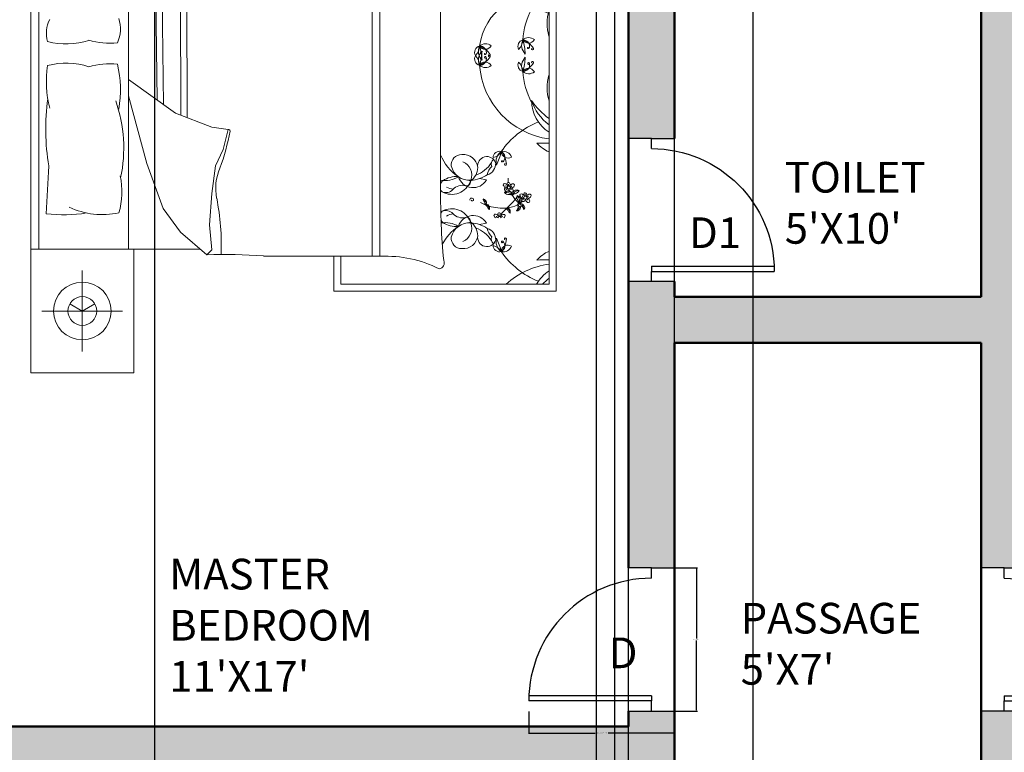
# Model space of a CAD drawing. Units: inches. Extents: x -55 to 413, y -498 to 86.
# Tile 4 of 6: x 45 to 238, y -201 to -57. Entities that reach past the tile are written whole.
import ezdxf

# ---------------------------------------------------------------- set-up
doc = ezdxf.new("R2010")
doc.units = ezdxf.units.IN
doc.header["$MEASUREMENT"] = 0
for name, color, linetype, lineweight in [('A-ANNO-DIMS', 2, 'Continuous', 18), ('A-ANNO-TEXT', 7, 'Continuous', 25), ('A-AREA-IDEN', 7, 'Continuous', 25), ('A-DOOR', 3, 'Continuous', 25), ('A-FURN', 9, 'Continuous', 18), ('A-WALL', 7, 'Continuous', 50), ('A-WALL-PATT', 8, 'Continuous', 13)]:
    doc.layers.add(name, color=color, linetype=linetype, lineweight=lineweight)
doc.styles.get("Standard").update_dxf_attribs({"font": 'arial.ttf'})
doc.dimstyles.get("Standard").update_dxf_attribs({"dimtxt": 0.18, "dimasz": 0.18, "dimexe": 0.18, "dimexo": 0.0625, "dimgap": 0.09, "dimtad": 0, "dimtih": 1, "dimtoh": 1, "dimdec": 0, "dimzin": 0, "dimdsep": 46, "dimlunit": 3, "dimtxsty": 'Standard', "dimcen": 0.09, "dimadec": 0, "dimazin": 0, "dimtfac": 1, "dimtdec": 0, "dimtofl": 0, "dimtmove": 0, "dimatfit": 3, "dimfxl": 1, "dimtolj": 1, "dimtzin": 0, "dimarcsym": 0})

# ---------------------------------------------------------------- blocks, each defined once
blk = doc.blocks.new('BED-DOUBLE-WITH-NIGHTSTANDS')
for p, q in [((0, 0), (0, 120.84)), ((10.07, 100.86), (10.07, 116.65)), ((17.96, 108.75), (2.18, 108.75)), ((59.24, 97.34), (59.24, 104.05)), ((59.24, 104.05), (102.77, 104.05)), ((102.77, 104.05), (102.77, 15.95)), ((60.64, 102.65), (60.64, 97.32)), ((101.37, 102.65), (60.64, 102.65)), ((101.37, 17.35), (101.37, 102.65)), ((1.55, 96.67), (1.55, 24.17)), ((19.1, 24.17), (19.1, 96.67)), ((24.12, 96.35), (24.72, 53.32)), ((25.36, 96.3), (25.98, 52.42)), ((66.77, 97.22), (66.77, 22.78)), ((68.28, 97.33), (68.28, 22.78)), ((29.16, 96.24), (29.34, 50.35)), ((30.4, 96.24), (30.59, 49.88)), ((89.11, 90.74), (87.75, 91)), ((80.15, 84.95), (80.15, 35.89)), ((89.11, 82.29), (87.75, 82.03)), ((19.1, 57.36), (28.31, 50.74)), ((22.69, 40.95), (19.1, 54.13)), ((28.31, 50.74), (35.41, 48.05)), ((35.41, 48.05), (38.59, 47.56)), ((38.59, 47.56), (37.61, 43.64)), ((37.61, 43.64), (36.14, 40.46)), ((25.87, 32.14), (22.69, 40.95)), ((36.14, 40.46), (35.41, 35.08)), ((89.11, 37.7), (87.75, 37.97)), ((35.41, 35.08), (34.92, 28.96)), ((29.29, 27.49), (25.87, 32.14)), ((34.92, 28.96), (35.41, 24.06)), ((89.11, 29.26), (87.75, 28.99)), ((34.43, 23.09), (29.29, 27.49)), ((0, 24.17), (33.17, 24.17)), ((35.41, 24.06), (34.43, 23.09)), ((59.24, 15.95), (59.24, 22.78)), ((60.64, 22.78), (60.64, 17.35)), ((10.07, 19.98), (10.07, 4.19)), ((60.64, 17.35), (101.37, 17.35)), ((102.77, 15.95), (59.24, 15.95)), ((17.96, 12.08), (2.18, 12.08))]:
    blk.add_line(p, q)
for points in [[(0, 96.67), (20.14, 96.67), (20.14, 120.84), (0, 120.84)], [(10.07, 108.75), (7.63, 107.35)], [(10.07, 108.75), (12.51, 107.35)], [(20.14, 24.17), (20.14, 0), (0, 0)], [(10.07, 12.08), (7.63, 13.49)], [(10.07, 12.08), (12.51, 13.49)]]:
    blk.add_lwpolyline(points)
for points in [[(65.82, 97.19, 0.056112), (72.47, 98.06, 0.095341), (78.87, 99.76)], [(3.01, 89.73, -0.074897), (10.9, 89.58, 0.472817)], [(11.35, 65.01, -0.14099), (3.29, 64.77, -0.235245)], [(11.35, 59.85, 0.14099), (3.29, 60.09, 0.235245)], [(3.01, 31.11, 0.074897), (10.9, 31.25, -0.472817)], [(45.49, 22.83, 0.001242), (68.42, 22.78, -0.127202), (79.85, 20.35)]]:
    blk.add_lwpolyline(points, format="xyb")
for centre, radius in [((10.07, 108.75), 5.64), ((10.07, 108.75), 2.82), ((96.74, 85.77), 0.308), ((93.49, 83.76), 0.308), ((93.49, 36.24), 0.308), ((96.74, 34.23), 0.308), ((10.07, 12.08), 5.64), ((10.07, 12.08), 2.82)]:
    blk.add_circle(centre, radius)
for centre, radius, start, end in [((105.05, 87.4), 15.78, 111.4092, 145.6135), ((103.49, 114.39), 15.78, 228.1144, 262.255), ((105.6, 106.48), 7.69, 209.8884, 236.5383), ((107.04, 109.24), 9.58, 223.5186, 233.6964), ((79.49, 98.85), 1.1, 336.5219, 123.8264), ((197.68, 88.65), 117.59, 175.2402, 181.8035), ((33.86, 313.3), 217.13, 266.1, 270.9282), ((41.76, 379.4), 283.23, 269.1145, 274.8735), ((91.72, 95.04), 1.31, 76.272, 177.0484), ((89.73, 97.71), 2.7, 284.7031, 328.6173), ((93.49, 94.28), 2.49, 125.7657, 194.5347), ((81.25, 98.7), 11.04, 332.8176, 347.4827), ((92.4, 94.6), 1.75, 20.9613, 102.2885), ((93.35, 96.35), 1.32, 181.7131, 301.5367), ((89.03, 93.68), 3.99, 2.0648, 41.1598), ((91.43, 95.17), 1.29, 316.2238, 62.3173), ((103.83, 102.17), 6.42, 221.0454, 247.4453), ((100.38, 119.75), 21.83, 266.3481, 272.5919), ((88.66, 99), 9.15, 203.6453, 236.3329), ((84.27, 93.67), 2.04, 88.9462, 185.5144), ((84.56, 92.84), 2.89, 7.1143, 95.0551), ((89.21, 93.5), 1.81, 19.1312, 189.736), ((91.18, 93.88), 1.11, 126.7319, 206.0245), ((92.17, 94.41), 0.103, 20.2667, 316.2271), ((85.78, 94.3), 3.63, 193.079, 274.7067), ((83.46, 91.7), 2.8, 338.5779, 68.4181), ((83.92, 93.34), 3.51, 305.9599, 357.6409), ((85.22, 97.1), 5.7, 288.2955, 328.7386), ((88.67, 93.94), 2.26, 285.6955, 4.031), ((91.68, 91.5), 2.41, 128.4175, 173.8338), ((92.82, 93.82), 0.196, 168.5166, 2.0648), ((92.72, 93.84), 0.0952, 52.0591, 168.5166), ((81.49, 89.45), 1.46, 127.675, 162.5814), ((81.04, 95.65), 5.01, 259.249, 301.1782), ((83.22, 86.74), 4.66, 85.2696, 124.215), ((86.51, 92.24), 3, 196.8663, 330.0915), ((83.22, 86.74), 4.66, 53.6555, 57.2989), ((85.68, 97.15), 6.48, 273.4924, 303.7117), ((-1146.98, 23.12), 1151.92, 2.85022, 3.31479), ((14.07, 74.34), 15.57, 78.2417, 114.8684), ((1.6, 85.42), 16.19, 348.9631, 14.8961), ((81.49, 89.45), 1.46, 196.6343, 225.5483), ((82.34, 91.77), 3.85, 240.8249, 340.7178), ((81.2, 90.06), 1.81, 246.1646, 318.4347), ((83.04, 92.35), 3.47, 240.0851, 262.564), ((84.4, 87.22), 2.48, 74.8529, 138.4347), ((85.25, 90.33), 0.75, 254.8529, 12.6959), ((90.82, 89.21), 0.238, 125.0752, 284.7644), ((91.19, 89.3), 0.513, 127.3642, 168.4363), ((90.79, 89.71), 0.74, 277.4968, 341.2737), ((91.37, 89.36), 0.294, 88.1325, 178.8919), ((91.96, 89.05), 0.636, 136.3462, 189.6513), ((91.6, 88.99), 0.265, 189.6513, 312.3208), ((91.66, 89.72), 0.308, 183.2768, 356.7232), ((92.63, 89.17), 1.01, 164.2829, 186.9148), ((91.44, 89.17), 0.504, 312.3208, 40.2111), ((92.5, 89.73), 0.715, 201.6382, 274.947), ((91.56, 88.75), 0.934, 42.3896, 66.5724), ((100.98, 96.15), 11.47, 217.9541, 226.8459), ((92.23, 89.3), 0.508, 10.9597, 52.2379), ((92.55, 89.26), 0.236, 274.947, 37.5263), ((94.05, 88.22), 0.634, 115.5379, 168.6744), ((91.9, 89.14), 1.91, 329.344, 349.7412), ((90.37, 88.7), 3.41, 352.8698, 1.6736), ((92.47, 77.79), 10.01, 110.1059, 116.9968), ((86.93, 87.31), 1.94, 336.3901, 344.4871), ((89.04, 86.81), 0.246, 83.9457, 185.6216), ((88.06, 87.04), 1.01, 328.836, 0.8141), ((88.58, 86.75), 0.58, 306.5232, 32.4668), ((89.27, 87.2), 0.246, 112.5583, 214.2343), ((89.11, 87.64), 0.58, 265.7131, 351.6568), ((88.6, 87.96), 1.01, 297.3659, 329.344), ((87.84, 88.83), 1.94, 313.6929, 321.7899), ((89.98, 87.5), 0.634, 115.5379, 168.6744), ((87.83, 88.42), 1.91, 329.344, 349.7412), ((92.47, 77.79), 10.01, 86.1723, 106.4158), ((86.31, 87.98), 3.41, 352.8698, 1.6736), ((93.34, 87.92), 0.246, 112.5583, 214.2343), ((93.18, 88.36), 0.58, 265.7131, 351.6568), ((92.67, 88.68), 1.01, 297.3659, 329.344), ((92.72, 82.78), 5.02, 60.7959, 85.244), ((82.04, 75.56), 16.51, 37.8256, 47.7588), ((91.9, 89.55), 1.94, 313.6929, 321.7899), ((99.38, 82.26), 6.02, 130.182, 149.456), ((95.16, 88.01), 0.344, 33.0979, 123.1364), ((87.59, 83.16), 8.99, 31.1156, 34.8118), ((94.67, 87.42), 0.93, 2.3172, 70.5201), ((94.22, 86.41), 1.4, 310.9365, 22.7695), ((95.43, 87.19), 0.268, 135.7354, 318.1297), ((94.99, 87.63), 0.356, 315.7354, 31.1156), ((94.69, 86.87), 0.826, 319.3812, 5.5456), ((95.64, 87.19), 0.268, 68.2452, 250.6395), ((95.02, 87.52), 0.801, 352.6008, 57.1845), ((97.88, 82.14), 5.36, 111.7087, 116.2181), ((92.72, 82.78), 5.02, 47.5083, 55.9967), ((95.78, 87.7), 0.801, 252.8042, 349.6943), ((95.02, 86.27), 0.853, 331.1838, 51.6792), ((95.87, 87.77), 0.356, 248.2452, 323.6254), ((95.55, 87.99), 0.93, 291.7087, 3.0299), ((88.91, 92.89), 8.99, 323.6254, 327.3216), ((96.29, 87.75), 0.344, 325.6077, 55.6462), ((97.67, 85.85), 0.97, 121.9501, 165.2442), ((97.31, 86.42), 0.305, 44.3732, 121.9501), ((82.34, 81.26), 3.85, 19.2822, 119.1751), ((81.2, 82.97), 1.81, 41.5653, 113.8354), ((86.24, 86.19), 0.379, 169.5864, 349.5616), ((86.38, 86.17), 0.233, 349.5616, 167.2949), ((89.11, 86.04), 0.634, 129.5056, 182.6421), ((87.29, 87.51), 1.91, 308.4388, 328.836), ((86.96, 89.06), 3.41, 296.5064, 305.3102), ((93.04, 86.11), 1.4, 253.6301, 325.4631), ((93.43, 84.17), 0.992, 82.0748, 142.6895), ((93.32, 85.53), 1.02, 228.342, 274.9894), ((93.35, 85.36), 0.853, 273.8774, 357.1501), ((93.68, 85.97), 0.826, 262.0748, 308.2393), ((95.01, 85.12), 0.853, 181.4625, 249.4747), ((94.87, 85.79), 0.826, 215.1128, 261.2773), ((95.53, 85.75), 1.4, 197.889, 269.722), ((94.59, 84), 0.992, 20.6625, 81.2773), ((96.07, 85.69), 0.992, 139.3812, 199.9959), ((94.86, 86.33), 1.02, 285.6484, 332.2957), ((95.89, 85.25), 0.238, 125.0752, 284.7644), ((96.26, 85.34), 0.513, 93.635, 168.4363), ((96.19, 86.16), 0.302, 138.2946, 276.2474), ((95.86, 85.76), 0.74, 277.4968, 341.2737), ((96.31, 86.11), 0.42, 358.5719, 143.8954), ((96.45, 85.41), 0.294, 88.1325, 178.8919), ((96.55, 86.44), 0.424, 208.8493, 269.9355), ((96.19, 86.34), 0.484, 274.2123, 318.1587), ((97.04, 85.1), 0.636, 136.3462, 189.6513), ((96.67, 85.04), 0.265, 189.6513, 312.3208), ((97.7, 85.22), 1.01, 164.2829, 186.9148), ((96.51, 85.21), 0.504, 312.3208, 40.2111), ((97.58, 85.78), 0.715, 201.6382, 274.947), ((97, 86.23), 0.204, 262.868, 7.094), ((96.63, 84.8), 0.934, 42.3896, 66.5724), ((96.97, 86.4), 0.607, 278.5614, 22.5914), ((97.31, 85.35), 0.508, 10.9597, 118.7804), ((97.62, 85.3), 0.236, 274.947, 37.5263), ((81.49, 83.58), 1.46, 134.4517, 156.7144), ((81.49, 83.58), 1.46, 203.2856, 232.325), ((83.04, 80.68), 3.47, 97.436, 119.9149), ((84.4, 85.81), 2.48, 221.5653, 285.1471), ((86.51, 80.79), 3, 29.9085, 163.1337), ((85.25, 82.7), 0.75, 347.3041, 105.1471), ((92.65, 83.24), 0.238, 125.0752, 284.7644), ((93.02, 83.33), 0.513, 93.635, 168.4363), ((92.95, 84.14), 0.302, 138.2946, 276.2474), ((92.61, 83.74), 0.74, 277.4968, 341.2737), ((93.06, 84.1), 0.42, 358.5719, 143.8954), ((93.2, 83.4), 0.294, 88.1325, 178.8919), ((93.31, 84.43), 0.424, 208.8493, 269.9355), ((92.95, 84.33), 0.484, 274.2123, 318.1587), ((93.79, 83.09), 0.636, 136.3462, 189.6513), ((93.43, 83.02), 0.265, 189.6513, 312.3208), ((94.45, 83.21), 1.01, 164.2829, 186.9148), ((94.42, 83.84), 0.97, 121.9501, 165.2442), ((93.27, 83.2), 0.504, 312.3208, 40.2111), ((94.33, 83.77), 0.715, 201.6382, 274.947), ((93.75, 84.21), 0.204, 262.868, 7.094), ((93.39, 82.79), 0.934, 42.3896, 66.5724), ((93.73, 84.38), 0.607, 278.5614, 22.5914), ((94.06, 83.34), 0.508, 10.9597, 118.7804), ((99.38, 82.26), 6.02, 156.1523, 156.9499), ((94.07, 84.4), 0.305, 44.3732, 121.9501), ((94.37, 83.29), 0.236, 274.947, 37.5263), ((95.09, 85.27), 1.02, 248.3627, 295.0101), ((2.79, 78.43), 15.38, 333.8761, 16.1746), ((81.04, 77.38), 5.01, 58.8218, 100.2867), ((88.66, 74.03), 9.15, 123.6671, 158.5059), ((83.22, 86.29), 4.66, 235.785, 274.7304), ((85.78, 78.73), 3.63, 85.2933, 166.921), ((83.46, 81.33), 2.8, 291.5819, 21.4221), ((83.22, 86.29), 4.66, 302.7011, 306.3445), ((83.92, 79.69), 3.51, 2.3591, 54.0401), ((85.68, 75.88), 6.48, 56.2883, 86.5076), ((85.22, 75.93), 5.7, 31.2614, 71.7045), ((91.68, 81.53), 2.41, 186.1662, 231.5825), ((88.67, 79.09), 2.26, 355.969, 74.3045), ((99.38, 82.26), 6.02, 175.2415, 182.8929), ((24.16, 75.39), 21.24, 166.3427, 191.1841), ((84.27, 79.36), 2.04, 174.4856, 271.0538), ((84.56, 80.19), 2.89, 264.9449, 352.8857), ((89.21, 79.53), 1.81, 170.264, 340.8688), ((91.18, 79.16), 1.11, 153.9755, 233.2681), ((93.49, 78.75), 2.49, 165.4653, 234.2343), ((81.25, 74.33), 11.04, 12.5173, 27.1824), ((89.03, 79.35), 3.99, 318.8402, 357.9352), ((92.82, 79.21), 0.196, 357.9352, 191.4834), ((92.72, 79.19), 0.0952, 191.4834, 307.9409), ((91.72, 77.99), 1.31, 182.9516, 283.728), ((89.73, 75.32), 2.7, 31.3827, 75.2969), ((91.43, 77.86), 1.29, 297.6827, 43.7762), ((93.35, 76.68), 1.32, 58.4633, 178.2869), ((92.4, 78.43), 1.75, 257.7115, 339.0387), ((92.24, 78.64), 0.171, 43.7762, 339.7183), ((105.05, 85.63), 15.78, 214.3865, 248.5908), ((103.83, 70.86), 6.42, 112.5547, 138.9546), ((100.38, 53.28), 21.83, 87.4081, 93.6519), ((99.85, 62.15), 12.21, 82.8636, 171.8197), ((100.7, 70.21), 2.83, 76.3898, 169.0739), ((100.31, 68.09), 3.58, 72.8609, 131.9049), ((111.94, 63.87), 15.78, 152.5854, 175.5377), ((98.73, 63.73), 7.06, 68.117, 96.6195), ((109.66, 68.29), 8.68, 162.9798, 196.4569), ((9.04, 66.43), 5.98, 153.3437, 196.1026), ((11.12, 67.24), 6.41, 335.0183, 18.5407), ((97.39, 63.8), 1.75, 50.8855, 132.2127), ((114.13, 64.85), 12.83, 174.3643, 175.6213), ((122.92, 58.09), 22.93, 160.0972, 160.2783), ((15.38, 79.26), 14.81, 254.1707, 275.9871), ((88.12, 62.64), 1.31, 106.1963, 206.9726), ((85.07, 63.96), 2.7, 314.6273, 358.5415), ((90.03, 62.87), 2.49, 155.6899, 224.4589), ((88.94, 62.6), 1.75, 50.8855, 132.2127), ((88.88, 64.58), 1.32, 211.6373, 331.4609), ((87.81, 62.6), 1.29, 346.148, 92.2415), ((86.47, 60.12), 3.99, 31.989, 71.0841), ((77.23, 60.59), 11.04, 2.7418, 17.407), ((96.58, 63.84), 1.31, 106.1963, 206.9726), ((93.52, 65.17), 2.7, 314.6273, 358.5415), ((98.49, 64.07), 2.49, 155.6899, 224.4589), ((97.33, 65.79), 1.32, 211.6373, 331.4609), ((94.92, 61.33), 3.99, 31.989, 71.0841), ((85.68, 61.8), 11.04, 2.7418, 17.407), ((96.26, 63.81), 1.29, 346.148, 92.2415), ((97.28, 63.53), 0.103, 50.1909, 346.0209), ((88.12, 61.39), 1.31, 153.0274, 253.8037), ((85.07, 60.06), 2.7, 1.4585, 45.3727), ((90.03, 61.16), 2.49, 135.5411, 204.3101), ((77.23, 63.43), 11.04, 342.593, 357.2582), ((86.47, 63.91), 3.99, 288.9159, 328.011), ((87.81, 61.42), 1.29, 267.7585, 13.852), ((88.83, 62.32), 0.103, 50.1909, 346.0209), ((88.9, 61.69), 0.171, 13.852, 309.9245), ((89.59, 62.1), 0.0952, 81.9833, 198.4408), ((89.59, 61.93), 0.0952, 161.5592, 278.0167), ((89.68, 62.13), 0.196, 198.4408, 31.989), ((89.68, 61.9), 0.196, 328.011, 161.5592), ((98.49, 59.95), 2.49, 135.5411, 204.3101), ((85.68, 62.23), 11.04, 342.593, 357.2582), ((98.14, 63.34), 0.196, 198.4408, 31.989), ((98.04, 63.3), 0.0952, 81.9833, 198.4408), ((24.59, 56.92), 21.53, 171.5249, 193.96), ((15.38, 45.61), 14.81, 84.0129, 105.8293), ((-3.78, 55.31), 21.31, 349.8617, 13.6238), ((88.88, 59.44), 1.32, 28.5391, 148.3627), ((88.94, 61.43), 1.75, 227.7873, 309.1145), ((103.49, 61.36), 15.78, 184.4623, 262.255), ((96.58, 60.18), 1.31, 153.0274, 253.8037), ((93.52, 58.85), 2.7, 1.4585, 45.3727), ((94.92, 62.7), 3.99, 288.9159, 328.011), ((96.26, 60.21), 1.29, 267.7585, 13.852), ((97.35, 60.48), 0.171, 13.852, 309.9245), ((98.14, 60.69), 0.196, 328.011, 161.5592), ((98.04, 60.72), 0.0952, 161.5592, 278.0167), ((97.33, 58.23), 1.32, 28.5391, 148.3627), ((97.39, 60.22), 1.75, 227.7873, 309.1145), ((111.94, 60.15), 15.78, 184.4623, 207.4146), ((109.66, 55.74), 8.68, 163.5431, 197.0202), ((114.13, 59.18), 12.83, 184.3787, 185.6357), ((122.92, 65.93), 22.93, 199.7217, 199.9028), ((46.74, 47.67), 43.83, 172.2196, 189.497), ((-9.91, 43.94), 28.09, 348.0397, 19.2615), ((105.6, 53.44), 7.69, 181.272, 236.5383), ((109.73, 61.24), 14.25, 214.0123, 234.053), ((107.04, 56.21), 9.58, 197.8504, 233.6964), ((105.05, 34.36), 15.78, 111.4092, 145.6135), ((-7.08, 55.95), 46.86, 340.1194, 349.3383), ((38.69, 47.29), 0.292, 358.8623, 109.7536), ((100.38, 66.71), 21.83, 266.3481, 272.5919), ((103.83, 49.14), 6.42, 221.0454, 247.4453), ((88.66, 45.97), 9.15, 201.4941, 236.3329), ((84.27, 40.64), 2.04, 88.9462, 185.5144), ((84.56, 39.8), 2.89, 7.1143, 95.0551), ((91.72, 42), 1.31, 76.272, 177.0484), ((89.73, 44.68), 2.7, 284.7031, 328.6173), ((93.49, 41.25), 2.49, 125.7657, 194.5347), ((81.25, 45.67), 11.04, 332.8176, 347.4827), ((92.4, 41.56), 1.75, 20.9613, 102.2885), ((91.43, 42.13), 1.29, 316.2238, 62.3173), ((89.03, 40.65), 3.99, 2.0648, 41.1598), ((93.35, 43.31), 1.32, 181.7131, 301.5367), ((83.46, 38.67), 2.8, 338.5779, 68.4181), ((85.22, 44.06), 5.7, 288.2955, 328.7386), ((89.21, 40.47), 1.81, 19.1312, 189.736), ((88.67, 40.9), 2.26, 285.6955, 4.031), ((91.18, 40.84), 1.11, 126.7319, 206.0245), ((92.17, 41.37), 0.103, 20.2667, 316.2271), ((92.82, 40.78), 0.196, 168.5166, 2.0648), ((92.72, 40.8), 0.0952, 52.0591, 168.5166), ((-1146.98, 97.71), 1151.92, 356.68521, 357.14978), ((1.6, 35.42), 16.19, 345.1039, 11.0369), ((46, 36.05), 9.84, 156.2616, 191.3392), ((85.78, 41.27), 3.63, 193.079, 274.7067), ((83.92, 40.3), 3.51, 305.9599, 357.6409), ((85.68, 44.12), 6.48, 273.4924, 303.7117), ((91.68, 38.46), 2.41, 128.4175, 173.8338), ((81.04, 42.61), 5.01, 259.7133, 301.1782), ((81.49, 36.41), 1.46, 127.675, 156.7144), ((82.34, 38.74), 3.85, 240.8249, 340.7178), ((83.22, 33.71), 4.66, 85.2696, 124.215), ((84.4, 34.18), 2.48, 74.8529, 138.4347), ((86.51, 39.2), 3, 196.8663, 330.0915), ((85.25, 37.3), 0.75, 254.8529, 12.6959), ((83.22, 33.71), 4.66, 53.6555, 57.2989), ((92.65, 36.76), 0.238, 75.2356, 234.9248), ((92.61, 36.25), 0.74, 18.7263, 82.5032), ((93.2, 36.6), 0.294, 181.1081, 271.8675), ((93.79, 36.91), 0.636, 170.3487, 223.6538), ((93.43, 36.97), 0.265, 47.6792, 170.3487), ((99.38, 37.73), 6.02, 177.1071, 184.7585), ((94.45, 36.79), 1.01, 173.0852, 195.7171), ((93.27, 36.8), 0.504, 319.7889, 47.6792), ((94.33, 36.23), 0.715, 85.053, 158.3618), ((94.37, 36.71), 0.236, 322.4737, 85.053), ((205.94, 34.45), 125.79, 179.3433, 185.6887), ((81.49, 36.41), 1.46, 203.229, 225.5483), ((81.2, 37.03), 1.81, 246.1646, 318.4347), ((83.04, 39.32), 3.47, 240.0851, 262.564), ((93.02, 36.66), 0.513, 191.5637, 266.365), ((93.32, 34.47), 1.02, 85.0106, 131.658), ((93.04, 33.88), 1.4, 34.5369, 106.3699), ((93.43, 35.83), 0.992, 217.3105, 277.9252), ((92.95, 35.85), 0.302, 83.7526, 221.7054), ((93.06, 35.9), 0.42, 216.1046, 1.4281), ((93.31, 35.57), 0.424, 90.0645, 151.1507), ((92.95, 35.67), 0.484, 41.8413, 85.7877), ((93.35, 34.63), 0.853, 2.8499, 86.1226), ((94.42, 36.16), 0.97, 194.7558, 238.0499), ((93.68, 34.03), 0.826, 51.7607, 97.9252), ((93.75, 35.78), 0.204, 352.906, 97.132), ((93.39, 37.21), 0.934, 293.4276, 317.6104), ((94.06, 36.66), 0.508, 241.2196, 349.0403), ((93.73, 35.61), 0.607, 337.4086, 81.4386), ((99.38, 37.73), 6.02, 203.0501, 203.8477), ((94.07, 35.59), 0.305, 238.0499, 315.6268), ((95.01, 34.88), 0.853, 110.5253, 178.5375), ((95.53, 34.25), 1.4, 90.278, 162.111), ((94.87, 34.2), 0.826, 98.7227, 144.8872), ((99.38, 37.73), 6.02, 210.544, 229.818), ((95.09, 34.73), 1.02, 64.9899, 111.6373), ((94.59, 36), 0.992, 278.7227, 339.3375), ((95.89, 34.74), 0.238, 75.2356, 234.9248), ((95.86, 34.24), 0.74, 18.7263, 82.5032), ((97.04, 34.9), 0.636, 170.3487, 223.6538), ((96.67, 34.96), 0.265, 47.6792, 170.3487), ((97.7, 34.78), 1.01, 173.0852, 195.7171), ((96.51, 34.78), 0.504, 319.7889, 47.6792), ((97.58, 34.22), 0.715, 85.053, 158.3618), ((97.62, 34.69), 0.236, 322.4737, 85.053), ((-8.36, 25.15), 45.61, 357.4519, 11.3392), ((86.24, 33.8), 0.379, 10.4384, 190.4136), ((86.38, 33.83), 0.233, 192.7051, 10.4384), ((92.47, 42.2), 10.01, 243.0032, 249.8941), ((87.29, 32.49), 1.91, 31.164, 51.5612), ((89.11, 33.95), 0.634, 177.3579, 230.4944), ((86.96, 30.93), 3.41, 54.6898, 63.4936), ((86.93, 32.69), 1.94, 15.5129, 23.6099), ((89.04, 33.18), 0.246, 174.3784, 276.0543), ((88.06, 32.95), 1.01, 359.1859, 31.164), ((88.58, 33.25), 0.58, 327.5332, 53.4768), ((89.27, 32.8), 0.246, 145.7657, 247.4417), ((89.11, 32.36), 0.58, 8.3432, 94.2869), ((88.6, 32.04), 1.01, 30.656, 62.6341), ((82.04, 44.44), 16.51, 312.2412, 322.1744), ((92.72, 37.22), 5.02, 274.756, 299.2041), ((96.07, 34.31), 0.992, 160.0041, 220.6188), ((94.22, 33.59), 1.4, 337.2305, 49.0635), ((94.86, 33.66), 1.02, 27.7043, 74.3516), ((95.43, 32.81), 0.268, 41.8703, 224.2646), ((94.69, 33.12), 0.826, 354.4544, 40.6188), ((95.64, 32.8), 0.268, 109.3605, 291.7548), ((97.88, 37.85), 5.36, 243.7819, 248.2913), ((92.72, 37.22), 5.02, 304.0033, 312.4917), ((95.02, 33.73), 0.853, 308.3208, 28.8162), ((95.78, 32.29), 0.801, 10.3057, 107.1958), ((96.26, 34.65), 0.513, 191.5637, 266.365), ((96.19, 33.84), 0.302, 83.7526, 221.7054), ((95.55, 32.01), 0.93, 356.9701, 68.2913), ((96.31, 33.89), 0.42, 216.1046, 1.4281), ((96.45, 34.58), 0.294, 181.1081, 271.8675), ((96.55, 33.56), 0.424, 90.0645, 151.1507), ((96.19, 33.66), 0.484, 41.8413, 85.7877), ((97.67, 34.14), 0.97, 194.7558, 238.0499), ((97, 33.77), 0.204, 352.906, 97.132), ((96.63, 35.19), 0.934, 293.4276, 317.6104), ((97.31, 34.65), 0.508, 241.2196, 349.0403), ((96.97, 33.6), 0.607, 337.4086, 81.4386), ((97.31, 33.58), 0.305, 238.0499, 315.6268), ((14.07, 46.5), 15.57, 245.1316, 281.7583), ((81.49, 30.55), 1.46, 134.4517, 153.558), ((82.34, 28.23), 3.85, 19.2822, 119.1751), ((81.2, 29.93), 1.81, 41.5653, 113.8354), ((83.04, 27.64), 3.47, 97.436, 119.9149), ((84.4, 32.78), 2.48, 221.5653, 285.1471), ((87.84, 31.17), 1.94, 38.2101, 46.3071), ((89.98, 32.49), 0.634, 191.3256, 244.4621), ((87.83, 31.58), 1.91, 10.2588, 30.656), ((92.47, 42.2), 10.01, 253.5842, 273.8277), ((86.31, 32.02), 3.41, 358.3264, 7.1302), ((90.82, 30.79), 0.238, 75.2356, 234.9248), ((90.79, 30.29), 0.74, 18.7263, 82.5032), ((91.96, 30.94), 0.636, 170.3487, 223.6538), ((91.6, 31.01), 0.265, 47.6792, 170.3487), ((92.63, 30.82), 1.01, 173.0852, 195.7171), ((91.44, 30.83), 0.504, 319.7889, 47.6792), ((92.5, 30.26), 0.715, 85.053, 158.3618), ((100.98, 23.85), 11.47, 133.1541, 142.0459), ((92.55, 30.74), 0.236, 322.4737, 85.053), ((93.34, 32.08), 0.246, 145.7657, 247.4417), ((93.18, 31.64), 0.58, 8.3432, 94.2869), ((92.67, 31.32), 1.01, 30.656, 62.6341), ((91.9, 30.45), 1.94, 38.2101, 46.3071), ((94.05, 31.77), 0.634, 191.3256, 244.4621), ((91.9, 30.86), 1.91, 10.2588, 30.656), ((90.37, 31.3), 3.41, 358.3264, 7.1302), ((94.67, 32.58), 0.93, 289.4799, 357.6828), ((87.59, 36.83), 8.99, 325.1882, 328.8844), ((95.16, 31.99), 0.344, 236.8636, 326.9021), ((94.99, 32.37), 0.356, 328.8844, 44.2646), ((95.02, 32.47), 0.801, 302.8155, 7.3992), ((95.87, 32.22), 0.356, 36.3746, 111.7548), ((88.91, 27.1), 8.99, 32.6784, 36.3746), ((96.29, 32.24), 0.344, 304.3538, 34.3923), ((81.49, 30.55), 1.46, 210.0293, 232.325), ((81.04, 24.35), 5.01, 58.8218, 99.1554), ((83.22, 33.25), 4.66, 235.785, 274.7304), ((85.78, 25.7), 3.63, 85.2933, 166.921), ((86.51, 27.76), 3, 29.9085, 163.1337), ((83.46, 28.29), 2.8, 291.5819, 21.4221), ((85.25, 29.66), 0.75, 347.3041, 105.1471), ((83.22, 33.25), 4.66, 302.7011, 306.3445), ((83.92, 26.66), 3.51, 2.3591, 54.0401), ((85.68, 22.84), 6.48, 56.2883, 86.5076), ((91.19, 30.7), 0.513, 191.5637, 232.6358), ((91.37, 30.63), 0.294, 181.1081, 271.8675), ((91.66, 30.27), 0.308, 3.2768, 176.7232), ((91.56, 31.24), 0.934, 293.4276, 317.6104), ((92.23, 30.69), 0.508, 307.7621, 349.0403), ((88.66, 20.99), 9.15, 123.6671, 153.2997), ((85.22, 22.9), 5.7, 31.2614, 71.7045), ((88.67, 26.06), 2.26, 355.969, 74.3045), ((91.68, 28.5), 2.41, 186.1662, 231.5825), ((84.27, 26.32), 2.04, 174.4856, 271.0538), ((84.56, 27.16), 2.89, 264.9449, 352.8857), ((89.21, 26.49), 1.81, 170.264, 340.8688), ((91.18, 26.12), 1.11, 153.9755, 233.2681), ((93.49, 25.71), 2.49, 165.4653, 234.2343), ((81.25, 21.29), 11.04, 12.5173, 27.1824), ((89.03, 26.31), 3.99, 318.8402, 357.9352), ((91.43, 24.83), 1.29, 297.6827, 43.7762), ((92.24, 25.6), 0.171, 43.7762, 339.7183), ((92.82, 26.18), 0.196, 357.9352, 191.4834), ((92.72, 26.16), 0.0952, 191.4834, 307.9409), ((37.43, -87.71), 110.84, 85.8294, 91.553), ((89.73, 22.28), 2.7, 31.3827, 75.2969), ((91.72, 24.96), 1.31, 182.9516, 283.728), ((93.35, 23.65), 1.32, 58.4633, 178.2869), ((92.4, 25.4), 1.75, 257.7115, 339.0387), ((105.05, 32.6), 15.78, 214.3865, 248.5908), ((103.83, 17.82), 6.42, 112.5547, 138.9546), ((79.77, 21.46), 1.11, 273.98, 27.3412), ((103.49, 5.6), 15.78, 97.745, 131.8856), ((100.38, 0.25), 21.83, 87.4081, 93.6519), ((105.6, 13.52), 7.69, 123.4617, 150.1116), ((107.04, 10.75), 9.58, 126.3036, 136.4814)]:
    blk.add_arc(centre, radius, start, end)
blk = doc.blocks.new('DOOR-SINGLE-24')
for p, q in [((24, 28), (19.5, 28)), ((24, 26), (24, 28)), ((24, 28), (28.5, 28)), ((24, 3), (0, 3)), ((24, 2), (0, 2)), ((24, 3), (24, 2)), ((24, 0), (24, 2)), ((19.5, 0), (28.5, 0))]:
    blk.add_line(p, q)
blk.add_arc((24, 2), 24, 90, 180)
blk = doc.blocks.new('*D17')
at = {"layer": 'A-ANNO-DIMS', "color": 0, "lineweight": -2, "transparency": 16777216}
for p, q in [((144.5, -192.52), (144.5, -196.92)), ((173, -192.52), (173, -196.92)), ((144.68, -196.74), (157.5, -196.74)), ((172.82, -196.74), (160.01, -196.74))]:
    blk.add_line(p, q, dxfattribs=at)
at = {"layer": 'A-ANNO-DIMS', "color": 0, "transparency": 16777216}
for points in [[(144.68, -196.71), (144.68, -196.77), (144.5, -196.74)], [(172.82, -196.71), (172.82, -196.77), (173, -196.74)]]:
    blk.add_solid(points, dxfattribs=at)
at = {"layer": 'Defpoints', "color": 0, "transparency": 16777216}
for p in [(144.5, -192.46), (173, -192.46), (173, -196.74)]:
    blk.add_point(p, dxfattribs=at)
at = {"layer": 'A-ANNO-DIMS', "color": 0, "transparency": 16777216, "insert": (158.75, -196.74), "char_height": 0.18, "attachment_point": 5}
blk.add_mtext('\\A1;DOOR 2\'-4 1/2" TYP.', dxfattribs=at)
blk = doc.blocks.new('*D18')
at = {"layer": 'A-ANNO-DIMS', "color": 0, "lineweight": -2, "transparency": 16777216}
for p, q in [((173.07, -164.46), (177.46, -164.46)), ((177.28, -164.64), (177.28, -178.28)), ((177.28, -192.28), (177.28, -178.64)), ((173.07, -192.46), (177.46, -192.46))]:
    blk.add_line(p, q, dxfattribs=at)
at = {"layer": 'A-ANNO-DIMS', "color": 0, "transparency": 16777216}
for points in [[(177.25, -164.64), (177.31, -164.64), (177.28, -164.46)], [(177.25, -192.28), (177.31, -192.28), (177.28, -192.46)]]:
    blk.add_solid(points, dxfattribs=at)
at = {"layer": 'Defpoints', "color": 0, "transparency": 16777216}
for p in [(173, -164.46), (177.28, -164.46), (173, -192.46)]:
    blk.add_point(p, dxfattribs=at)
at = {"layer": 'A-ANNO-DIMS', "color": 0, "transparency": 16777216, "insert": (177.28, -178.46), "char_height": 0.18, "attachment_point": 5}
blk.add_mtext('\\A1;2\'-4" TYP.', dxfattribs=at)
blk = doc.blocks.new('*D40')
at = {"layer": 'A-ANNO-DIMS', "color": 0, "lineweight": -2, "transparency": 16777216}
for p, q in [((157.71, -357.4), (157.71, 47.52)), ((157.89, 47.34), (160.32, 47.34)), ((163.82, 47.34), (161.39, 47.34)), ((164, -357.4), (164, 47.52))]:
    blk.add_line(p, q, dxfattribs=at)
at = {"layer": 'A-ANNO-DIMS', "color": 0, "transparency": 16777216}
for points in [[(157.89, 47.37), (157.89, 47.31), (157.71, 47.34)], [(163.82, 47.37), (163.82, 47.31), (164, 47.34)]]:
    blk.add_solid(points, dxfattribs=at)
at = {"layer": 'Defpoints', "color": 0, "transparency": 16777216}
for p in [(164, 47.34), (157.71, -357.46), (164, -357.46)]:
    blk.add_point(p, dxfattribs=at)
at = {"layer": 'A-ANNO-DIMS', "color": 0, "transparency": 16777216, "insert": (160.86, 47.34), "char_height": 0.18, "attachment_point": 5}
blk.add_mtext('\\A1;0\'-6 1/2"', dxfattribs=at)
blk = doc.blocks.new('*D41')
at = {"layer": 'A-ANNO-DIMS', "color": 0, "lineweight": -2, "transparency": 16777216}
for p, q in [((173, -357.4), (173, 47.52)), ((173.18, 47.34), (180.15, 47.34)), ((188.17, 47.34), (181.21, 47.34)), ((188.35, -357.4), (188.35, 47.52))]:
    blk.add_line(p, q, dxfattribs=at)
at = {"layer": 'A-ANNO-DIMS', "color": 0, "transparency": 16777216}
for points in [[(173.18, 47.37), (173.18, 47.31), (173, 47.34)], [(188.17, 47.37), (188.17, 47.31), (188.35, 47.34)]]:
    blk.add_solid(points, dxfattribs=at)
at = {"layer": 'Defpoints', "color": 0, "transparency": 16777216}
for p in [(188.35, 47.34), (173, -357.46), (188.35, -357.46)]:
    blk.add_point(p, dxfattribs=at)
at = {"layer": 'A-ANNO-DIMS', "color": 0, "transparency": 16777216, "insert": (180.68, 47.34), "char_height": 0.18, "attachment_point": 5}
blk.add_mtext('\\A1;1\'-3 1/2"', dxfattribs=at)
blk = doc.blocks.new('*D43')
at = {"layer": 'A-ANNO-DIMS', "color": 0, "lineweight": -2, "transparency": 16777216}
for p, q in [((71.33, -456.4), (71.33, 47.52)), ((71.51, 47.34), (116, 47.34)), ((161.15, 47.34), (116.66, 47.34)), ((161.33, -456.4), (161.33, 47.52))]:
    blk.add_line(p, q, dxfattribs=at)
at = {"layer": 'A-ANNO-DIMS', "color": 0, "transparency": 16777216}
for points in [[(71.51, 47.37), (71.51, 47.31), (71.33, 47.34)], [(161.15, 47.37), (161.15, 47.31), (161.33, 47.34)]]:
    blk.add_solid(points, dxfattribs=at)
at = {"layer": 'Defpoints', "color": 0, "transparency": 16777216}
for p in [(161.33, 47.34), (71.33, -456.46), (161.33, -456.46)]:
    blk.add_point(p, dxfattribs=at)
at = {"layer": 'A-ANNO-DIMS', "color": 0, "transparency": 16777216, "insert": (116.33, 47.34), "char_height": 0.18, "attachment_point": 5}
blk.add_mtext('\\A1;7\'-6"', dxfattribs=at)

msp = doc.modelspace()

# ---------------------------------------------------------------- hatches: boundary and pattern name
at = {"layer": 'A-WALL-PATT'}
h = msp.add_hatch(color=256, dxfattribs=at)
h.dxf.hatch_style = 1
h.paths.add_polyline_path([(97.55, 17.54), (23, 17.54), (23, -94.08), (32, -94.08), (32, 8.54), (97.55, 8.54)])
h.paths.add_polyline_path([(191, 17.54), (157.55, 17.54), (157.55, 8.54), (164, 8.54), (164, -80.46), (168.5, -80.46), (173, -80.46), (173, 8.54), (191, 8.54)])
h.paths.add_polyline_path([(312.03, 17.54), (215, 17.54), (215, 8.54), (233, 8.54), (233, -111.46), (173, -111.46), (173, -108.46), (164, -108.46), (164, -164.46), (168.5, -164.46), (173, -164.46), (173, -120.46), (233, -120.46), (233, -164.46), (237.5, -164.46), (242, -164.46), (242, 8.54), (312.03, 8.54)])
h.paths.add_polyline_path([(383, 17.54), (372.03, 17.54), (372.03, 8.54), (374, 8.54), (374, -99.01), (383, -99.01)])
h.paths.add_polyline_path([(383, -159.01), (374, -159.01), (374, -195.46), (242, -195.46), (242, -192.46), (233, -192.46), (233, -204.46), (374, -204.46), (374, -224.71), (383, -224.71)])
h.paths.add_polyline_path([(173, -192.46), (164, -192.46), (164, -195.46), (32, -195.46), (32, -154.08), (23, -154.08), (23, -213.4), (32, -213.4), (32, -204.46), (164, -204.46), (164, -221.46), (168.5, -221.46), (173, -221.46)])
h.paths.add_polyline_path([(173, -249.46), (164, -249.46), (164, -252.46), (32, -252.46), (32, -237.4), (23, -237.4), (23, -273.22), (32, -273.22), (32, -261.46), (164, -261.46), (173, -261.46)])
h.paths.add_polyline_path([(32, -309.22), (23, -309.22), (23, -456.46), (23, -460.96), (199.52, -460.96), (199.52, -456.46), (32, -456.46), (32, -366.46), (97.71, -366.46), (97.71, -357.46), (32, -357.46)])
h.paths.add_polyline_path([(188.35, -357.46), (173, -357.46), (173, -302.07), (164, -302.07), (164, -357.46), (157.71, -357.46), (157.71, -366.46), (188.35, -366.46)])
h.paths.add_polyline_path([(223.25, -357.46), (212.35, -357.46), (212.35, -366.46), (223.25, -366.46), (223.25, -361.96)])
h.paths.add_polyline_path([(287.63, -357.46), (271.25, -357.46), (271.25, -361.96), (271.25, -366.46), (287.63, -366.46)])
h.paths.add_polyline_path([(374, -357.46), (311.63, -357.46), (311.63, -366.46), (374, -366.46)])
h.paths.add_polyline_path([(383, -456.46), (383, -366.46), (378.5, -366.46), (378.5, -456.46), (309.45, -456.46), (309.45, -460.96), (383, -460.96)])
h.paths.add_polyline_path([(309.45, -458.71), (199.52, -458.71), (199.52, -460.96), (309.45, -460.96)])
h.paths.add_polyline_path([(383, -260.71), (374, -260.71), (374, -280.96), (371, -280.96), (371, -285.46), (374, -285.46), (374, -366.46), (383, -366.46)])
h.paths.add_polyline_path([(343, -283.21), (343, -280.96), (321.5, -280.96), (321.5, -357.46), (326, -357.46), (326, -285.46), (343, -285.46)])

# ---------------------------------------------------------------- linework, layer by layer
at = {"layer": 'A-WALL'}
for p, q in [((164, 8.54), (164, -164.46)), ((173, 8.54), (173, -80.46)), ((233, 8.54), (233, -111.46)), ((173, -108.46), (173, -111.46)), ((173, -111.46), (233, -111.46)), ((173, -120.46), (233, -120.46)), ((173, -120.46), (173, -357.46)), ((233, -120.46), (233, -204.46)), ((164, -192.46), (164, -195.46)), ((32, -195.46), (164, -195.46))]:
    msp.add_line(p, q, dxfattribs=at)

# ---------------------------------------------------------------- block references
at = {"layer": 'A-DOOR', "extrusion": (0, 0, -1), "zscale": -1}
for p in [(-192.5, -108.46), (-261.5, -192.46)]:
    msp.add_blockref('DOOR-SINGLE-24', p, dxfattribs=at)
at = {"layer": 'A-DOOR'}
msp.add_blockref('DOOR-SINGLE-24', (144.5, -192.46), dxfattribs=at)
at = {"layer": 'A-FURN'}
msp.add_blockref('BED-DOUBLE-WITH-NIGHTSTANDS', (47.09, -126.29), dxfattribs=at)

# ---------------------------------------------------------------- texts
at = {"layer": 'A-ANNO-TEXT', "char_height": 6, "attachment_point": 1}
for s, insert in [('D1', (175.83, -95.9)), ('D', (160.12, -178.06))]:
    msp.add_mtext(s, dxfattribs=dict(at, insert=insert))
at = {"layer": 'A-AREA-IDEN', "char_height": 6, "attachment_point": 1}
for s, insert in [("TOILET\\P5'X10'", (194.57, -85.05)), ("MASTER\\PBEDROOM\\P11'X17'", (74.17, -162.66)), ("PASSAGE\\P5'X7'", (185.94, -171.28))]:
    msp.add_mtext(s, dxfattribs=dict(at, insert=insert))

# ---------------------------------------------------------------- dimensions: what is measured, and where the dimension line sits
at = {"layer": 'A-ANNO-DIMS'}
for base, p1, p2, picture, middle in [((161.33, 47.34), (71.33, -456.46), (161.33, -456.46), '*D43', (116.33, 47.34)), ((164, 47.34), (157.71, -357.46), (164, -357.46), '*D40', (160.86, 47.34)), ((188.3509, 47.3397), (173.0027, -357.4603), (188.3509, -357.4603), '*D41', (180.6768, 47.3397))]:
    dim = msp.add_linear_dim(base=base, p1=p1, p2=p2, dimstyle='Standard', override={"dimdec": 1, "dimlfac": 1, "dimrnd": 0, "dimzin": 1, "dimdsep": 46, "dimlunit": 4, "dimfrac": 2}, dxfattribs=at)
    dim.commit()
    dim.dimension.update_dxf_attribs({"geometry": picture, "text_midpoint": middle})
dim = msp.add_linear_dim(base=(177.28, -164.46), p1=(173, -192.46), p2=(173, -164.46), angle=90, text='<> TYP.', dimstyle='Standard', override={"dimdec": 1, "dimlfac": 1, "dimrnd": 0, "dimzin": 1, "dimdsep": 46, "dimlunit": 4, "dimfrac": 2}, dxfattribs=at)
dim.commit()
dim.dimension.update_dxf_attribs({"geometry": '*D18', "text_midpoint": (177.28, -178.46)})
dim = msp.add_linear_dim(base=(173, -196.74), p1=(144.5, -192.46), p2=(173, -192.46), text='DOOR <> TYP.', dimstyle='Standard', override={"dimdec": 1, "dimlfac": 1, "dimrnd": 0, "dimzin": 1, "dimdsep": 46, "dimlunit": 4, "dimfrac": 2}, dxfattribs=at)
dim.commit()
dim.dimension.update_dxf_attribs({"geometry": '*D17', "text_midpoint": (158.75, -196.74)})

doc.saveas('drawing.dxf')
